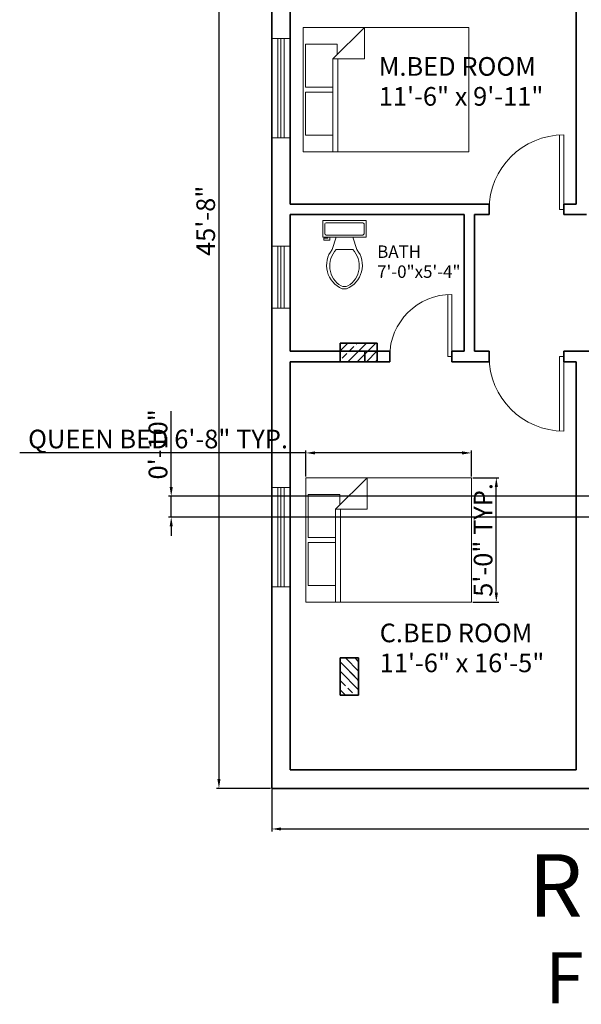
# Model space of a CAD drawing. Units: inches. Extents: x 2081 to 4786, y 1256 to 3802.
# Tile 1 of 7: x 2081 to 2352, y 1329 to 1804. Entities that reach past the tile are written whole.
import ezdxf

# ---------------------------------------------------------------- set-up
doc = ezdxf.new("R2010")
doc.units = ezdxf.units.IN
for name, color, linetype, lineweight in [('A-ANNO-DIMS', 18, 'Continuous', 18), ('A-ANNO-TITL', 18, 'Continuous', 35), ('A-AREA-IDEN', 18, 'Continuous', 18), ('A-COLS', 1, 'Continuous', 35), ('A-DOOR', 5, 'Continuous', 18), ('A-FLOR-FIXT', 18, 'Continuous', 18), ('A-FURN', 5, 'Continuous', 18), ('A-GLAZ', 11, 'Continuous', 18), ('A-WALL', 7, 'Continuous', 35)]:
    doc.layers.add(name, color=color, linetype=linetype, lineweight=lineweight)
doc.styles.get("Standard").update_dxf_attribs({"font": 'arial.ttf'})
doc.dimstyles.new('ISO-25', dxfattribs={"dimtxt": 9, "dimasz": 4.5, "dimexe": 1.25, "dimexo": 0.625, "dimtad": 1, "dimdec": 0, "dimlunit": 3, "dimtxsty": 'Standard', "dimcen": 2.5, "dimadec": 0, "dimazin": 0, "dimtfac": 1, "dimtdec": 0, "dimtmove": 0, "dimatfit": 3, "dimfxl": 1, "dimarcsym": 0})
pattern_1 = [(135, (1916.44, -3174.735), (-13.47038, -13.47038), []), (135, (1916.44, -3170.245), (-13.47038, -13.47038), []), (135, (1916.44, -3165.755), (-13.47038, -13.47038), []), (135, (1916.44, -3161.265), (-13.47038, -13.47038), [])]

# ---------------------------------------------------------------- blocks, each defined once
blk = doc.blocks.new('Bed - Queen')
for p, q in [((0, -80.00003), (0, 0)), ((0, 0), (59.99999, 0)), ((59.99999, 0), (59.99999, -80.00003)), ((7.99999, -1.2), (28.79998, -1.2)), ((7.99999, -14.4), (7.99999, -1.2)), ((28.79998, -1.2), (28.79998, -14.4)), ((31.19999, -1.2), (51.99999, -1.2)), ((31.19999, -14.4), (31.19999, -1.2)), ((51.99999, -1.2), (51.99999, -16.4)), ((0, -14.4), (44.8, -14.4)), ((44.8, -16.8), (0, -16.8)), ((59.99999, -29.6), (44.8, -14.4)), ((44.8, -14.4), (44.8, -29.6)), ((51.99999, -16.4), (46.79936, -16.4)), ((44.8, -29.6), (59.99999, -29.6)), ((59.99999, -80.00003), (0, -80.00003))]:
    blk.add_line(p, q)
blk = doc.blocks.new('Toilet - top')
for p, q in [((9.5, -6), (9.5, -2)), ((-10, -8.5), (-8, -8.5)), ((-10, -9.5), (-10, -8.5)), ((-7, -9.5), (-10, -9.5)), ((-8, -8.5), (-8, -8)), ((-7, -8), (-7, -9.5)), ((-4, -8), (-6, -14)), ((4, -8), (6, -14)), ((4, -14), (-4, -14))]:
    blk.add_line(p, q)
blk.add_lwpolyline([(10.5, -8), (10.5, 0), (-10.5, 0), (-10.5, -8)], close=True)
for points in [[(-9.5, -2), (-9.5, -6)], [(8.5, -1), (-8.5, -1)], [(-8.5, -7), (8.5, -7)]]:
    blk.add_lwpolyline(points)
for centre, radius, start, end in [((-8.62, -1.88), 0.884, 81.8699, 188.1301), ((8.62, -1.88), 0.884, 351.8699, 98.1301), ((-8.62, -6.12), 0.884, 171.8699, 278.1301), ((8.62, -6.12), 0.884, 261.8699, 8.1301), ((3.52, -21.58), 12.17, 141.4691, 247.9714), ((4.2, -21.82), 11.33, 136.3677, 238.9468), ((-3.52, -21.58), 12.17, 292.0284, 38.5307), ((-4.2, -21.82), 11.33, 301.053, 43.6321), ((0, -27.88), 4, 245.7318, 294.2682), ((0, -29), 4, 254.8605, 285.1395)]:
    blk.add_arc(centre, radius, start, end)
blk = doc.blocks.new('*D25')
at = {"layer": 'A-ANNO-DIMS', "color": 0, "lineweight": -2, "transparency": 16777216}
for p, q in [((2202.36, 1981.17), (2176.26, 1981.17)), ((2177.51, 1976.67), (2177.51, 1437.67)), ((2202.36, 1433.17), (2176.26, 1433.17))]:
    blk.add_line(p, q, dxfattribs=at)
at = {"layer": 'A-ANNO-DIMS', "color": 0, "transparency": 16777216}
for points in [[(2176.76, 1976.67), (2178.26, 1976.67), (2177.51, 1981.17)], [(2176.76, 1437.67), (2178.26, 1437.67), (2177.51, 1433.17)]]:
    blk.add_solid(points, dxfattribs=at)
at = {"layer": 'Defpoints', "color": 0, "transparency": 16777216}
for p in [(2202.98, 1981.17), (2177.51, 1433.17), (2202.98, 1433.17)]:
    blk.add_point(p, dxfattribs=at)
at = {"layer": 'A-ANNO-DIMS', "color": 0, "transparency": 16777216, "insert": (2172.29, 1707.17), "char_height": 9, "attachment_point": 5, "rotation": 90}
blk.add_mtext('45\'-8"', dxfattribs=at)
blk = doc.blocks.new('*D26')
at = {"layer": 'A-ANNO-DIMS', "color": 0, "lineweight": -2, "transparency": 16777216}
for p, q in [((2202.98, 1432.55), (2202.98, 1412.32)), ((3062.98, 1432.55), (3062.98, 1412.32)), ((2207.48, 1413.57), (3058.48, 1413.57))]:
    blk.add_line(p, q, dxfattribs=at)
at = {"layer": 'A-ANNO-DIMS', "color": 0, "transparency": 16777216}
for points in [[(2207.48, 1414.32), (2207.48, 1412.82), (2202.98, 1413.57)], [(3058.48, 1414.32), (3058.48, 1412.82), (3062.98, 1413.57)]]:
    blk.add_solid(points, dxfattribs=at)
at = {"layer": 'Defpoints', "color": 0, "transparency": 16777216}
for p in [(2202.98, 1433.17), (3062.98, 1433.17), (3062.98, 1413.57)]:
    blk.add_point(p, dxfattribs=at)
at = {"layer": 'A-ANNO-DIMS', "color": 0, "transparency": 16777216, "insert": (2632.98, 1418.79), "char_height": 9, "attachment_point": 5}
blk.add_mtext('71\'-8"', dxfattribs=at)
blk = doc.blocks.new('DOOR-SINGLE-36IN')
for p, q in [((34, 36), (34, 0)), ((36, 36), (36, 0)), ((36, 0), (34, 0))]:
    blk.add_line(p, q)
blk.add_arc((36, 0), 36, 90, 180)
blk = doc.blocks.new('DOOR-SINGLE-30IN')
for p, q in [((0, 30), (30, 30)), ((30, 30), (30, 28)), ((0, 28), (30, 28))]:
    blk.add_line(p, q)
blk.add_arc((30, 30), 30, 180, 270)
blk = doc.blocks.new('WINDOW-48IN')
for p, q in [((0, 0), (0, 9)), ((0, 9), (4, 9)), ((48, 6), (0, 6)), ((4, 9), (48, 9)), ((48, 0), (48, 9)), ((48, 4.5), (0, 4.5)), ((48, 3), (0, 3)), ((48, 0), (0, 0))]:
    blk.add_line(p, q)
blk = doc.blocks.new('WINDOW-30IN')
for p, q in [((0, 0), (0, 30)), ((0, 30), (9, 30)), ((3, 0), (3, 30)), ((4.5, 0), (4.5, 30)), ((6, 0), (6, 30)), ((9, 30), (9, 0)), ((9, 0), (0, 0))]:
    blk.add_line(p, q)
blk = doc.blocks.new('COLUMN-9X18IN')
h = blk.add_hatch()
h.set_pattern_fill('ANSI34', color=256, angle=90)
h.set_pattern_definition(pattern_1)
h.paths.add_polyline_path([(9, 18), (0, 18), (0, 0), (9, 0)])
h = blk.add_hatch()
h.set_pattern_fill('ANSI34', color=256, angle=90)
h.set_pattern_definition(pattern_1)
h.paths.add_polyline_path([(9, 18), (0, 18), (0, 0), (9, 0)])
h = blk.add_hatch()
h.set_pattern_fill('ANSI34', color=256, angle=90)
h.set_pattern_definition(pattern_1)
h.paths.add_polyline_path([(9, 18), (0, 18), (0, 0), (9, 0)])
h = blk.add_hatch()
h.set_pattern_fill('ANSI33', color=256, angle=90)
h.set_pattern_definition([(135, (1916.44, -3174.7355), (-4.490128, -4.490128), []), (135, (1916.44, -3170.2454), (-4.490128, -4.490128), [3.175, -1.5875])])
h.paths.add_polyline_path([(0, 0), (9, 0), (9, 18), (0, 18)])
for p, q in [((0, 0), (0, 18)), ((0, 18), (9, 18)), ((9, 18), (9, 0)), ((9, 0), (0, 0))]:
    blk.add_line(p, q)
blk = doc.blocks.new('*D37')
at = {"layer": 'A-ANNO-DIMS', "color": 0, "lineweight": -2, "transparency": 16777216}
for p, q in [((2219.45, 1595.12), (2081.31, 1595.12)), ((2219.45, 1583.74), (2219.45, 1596.37)), ((2294.95, 1595.12), (2223.95, 1595.12)), ((2299.45, 1583.74), (2299.45, 1596.37))]:
    blk.add_line(p, q, dxfattribs=at)
at = {"layer": 'A-ANNO-DIMS', "color": 0, "transparency": 16777216}
for points in [[(2223.95, 1595.87), (2223.95, 1594.37), (2219.45, 1595.12)], [(2294.95, 1595.87), (2294.95, 1594.37), (2299.45, 1595.12)]]:
    blk.add_solid(points, dxfattribs=at)
at = {"layer": 'Defpoints', "color": 0, "transparency": 16777216}
for p in [(2219.45, 1595.12), (2219.45, 1583.12), (2299.45, 1583.12)]:
    blk.add_point(p, dxfattribs=at)
at = {"layer": 'A-ANNO-DIMS', "color": 0, "transparency": 16777216, "insert": (2148.13, 1600.67), "char_height": 9, "attachment_point": 5}
blk.add_mtext('QUEEN BED 6\'-8" TYP.', dxfattribs=at)
blk = doc.blocks.new('*D38')
at = {"layer": 'A-ANNO-DIMS', "color": 0, "lineweight": -2, "transparency": 16777216}
for p, q in [((2300.08, 1583.12), (2312.7, 1583.12)), ((2311.45, 1527.62), (2311.45, 1578.62)), ((2300.08, 1523.12), (2312.7, 1523.12))]:
    blk.add_line(p, q, dxfattribs=at)
at = {"layer": 'A-ANNO-DIMS', "color": 0, "transparency": 16777216}
for points in [[(2310.7, 1578.62), (2312.2, 1578.62), (2311.45, 1583.12)], [(2310.7, 1527.62), (2312.2, 1527.62), (2311.45, 1523.12)]]:
    blk.add_solid(points, dxfattribs=at)
at = {"layer": 'Defpoints', "color": 0, "transparency": 16777216}
for p in [(2299.45, 1583.12), (2311.45, 1583.12), (2299.45, 1523.12)]:
    blk.add_point(p, dxfattribs=at)
at = {"layer": 'A-ANNO-DIMS', "color": 0, "transparency": 16777216, "insert": (2306.23, 1553.12), "char_height": 9, "attachment_point": 5, "rotation": 90}
blk.add_mtext('5\'-0" TYP.', dxfattribs=at)
blk = doc.blocks.new('*D60')
at = {"layer": 'A-ANNO-DIMS', "color": 0, "lineweight": -2, "transparency": 16777216}
for p, q in [((2358.89, 1801.88), (2358.89, 1811.5)), ((2380.23, 1801.88), (2380.23, 1811.5)), ((2358.89, 1810.25), (2278.16, 1810.25)), ((2375.73, 1810.25), (2363.39, 1810.25))]:
    blk.add_line(p, q, dxfattribs=at)
at = {"layer": 'A-ANNO-DIMS', "color": 0, "transparency": 16777216}
for points in [[(2363.39, 1811), (2363.39, 1809.5), (2358.89, 1810.25)], [(2375.73, 1811), (2375.73, 1809.5), (2380.23, 1810.25)]]:
    blk.add_solid(points, dxfattribs=at)
at = {"layer": 'Defpoints', "color": 0, "transparency": 16777216}
for p in [(2358.89, 1810.25), (2358.89, 1801.25), (2380.23, 1801.25)]:
    blk.add_point(p, dxfattribs=at)
at = {"layer": 'A-ANNO-DIMS', "color": 0, "transparency": 16777216, "insert": (2316.28, 1815.53), "char_height": 9, "attachment_point": 5}
blk.add_mtext('1\'-9 1/2" TYP.', dxfattribs=at)
blk = doc.blocks.new('*D81')
at = {"layer": 'A-ANNO-DIMS', "color": 0, "lineweight": -2, "transparency": 16777216}
for p, q in [((2154.48, 1578.67), (2154.48, 1615.34)), ((2684.36, 1574.17), (2153.23, 1574.17)), ((2154.48, 1564.17), (2154.48, 1574.17)), ((2684.36, 1564.17), (2153.23, 1564.17)), ((2154.48, 1559.67), (2154.48, 1555.17))]:
    blk.add_line(p, q, dxfattribs=at)
at = {"layer": 'A-ANNO-DIMS', "color": 0, "transparency": 16777216}
for points in [[(2153.73, 1578.67), (2155.23, 1578.67), (2154.48, 1574.17)], [(2153.73, 1559.67), (2155.23, 1559.67), (2154.48, 1564.17)]]:
    blk.add_solid(points, dxfattribs=at)
at = {"layer": 'Defpoints', "color": 0, "transparency": 16777216}
for p in [(2154.48, 1574.17), (2684.98, 1574.17), (2684.98, 1564.17)]:
    blk.add_point(p, dxfattribs=at)
at = {"layer": 'A-ANNO-DIMS', "color": 0, "transparency": 16777216, "insert": (2149.26, 1599.26), "char_height": 9, "attachment_point": 5, "rotation": 90}
blk.add_mtext('0\'-10"', dxfattribs=at)

msp = doc.modelspace()

# ---------------------------------------------------------------- linework, layer by layer
at = {"layer": 'A-WALL'}
for p, q in [((2202.98, 1981.17), (2202.98, 1433.17)), ((2211.98, 1715.17), (2211.98, 1834.17)), ((2349.98, 1715.17), (2349.98, 1834.17)), ((2211.98, 1715.17), (2307.98, 1715.17)), ((2307.98, 1710.17), (2307.98, 1715.17)), ((2343.98, 1710.17), (2343.98, 1715.17)), ((2343.98, 1715.17), (2349.98, 1715.17)), ((2211.98, 1710.17), (2295.98, 1710.17)), ((2211.98, 1644.17), (2211.98, 1710.17)), ((2295.98, 1644.17), (2295.98, 1710.17)), ((2300.98, 1644.17), (2300.98, 1710.17)), ((2300.98, 1710.17), (2307.98, 1710.17)), ((2343.98, 1710.17), (2354.98, 1710.17)), ((2211.98, 1644.17), (2259.98, 1644.17)), ((2247.98, 1639.17), (2247.98, 1644.17)), ((2259.98, 1644.17), (2259.98, 1639.17)), ((2289.98, 1639.17), (2289.98, 1644.17)), ((2289.98, 1644.17), (2295.98, 1644.17)), ((2300.98, 1644.17), (2307.98, 1644.17)), ((2307.98, 1639.17), (2307.98, 1644.17)), ((2343.98, 1639.17), (2343.98, 1644.17)), ((2343.98, 1644.17), (2429.98, 1644.17)), ((2211.98, 1442.17), (2211.98, 1639.17)), ((2211.98, 1639.17), (2259.98, 1639.17)), ((2289.98, 1639.17), (2307.98, 1639.17)), ((2343.98, 1639.17), (2349.98, 1639.17)), ((2349.98, 1442.17), (2349.98, 1639.17)), ((2349.98, 1442.17), (2211.98, 1442.17)), ((3062.98, 1433.17), (2202.98, 1433.17))]:
    msp.add_line(p, q, dxfattribs=at)

# ---------------------------------------------------------------- block references
at = {"layer": 'A-COLS', "rotation": 269.9999999999957}
msp.add_blockref('COLUMN-9X18IN', (2235.98, 1648.17), dxfattribs=at)
at = {"layer": 'A-COLS'}
msp.add_blockref('COLUMN-9X18IN', (2235.98, 1478.17), dxfattribs=at)
at = {"layer": 'A-DOOR'}
msp.add_blockref('DOOR-SINGLE-36IN', (2307.98, 1712.67), dxfattribs=at)
at = {"layer": 'A-DOOR', "rotation": 270}
msp.add_blockref('DOOR-SINGLE-30IN', (2259.98, 1671.67), dxfattribs=at)
at = {"layer": 'A-DOOR', "extrusion": (0, 0, -1), "zscale": -1, "rotation": 180}
msp.add_blockref('DOOR-SINGLE-36IN', (-2307.98, 1641.67), dxfattribs=at)
at = {"layer": 'A-FLOR-FIXT'}
msp.add_blockref('Toilet - top', (2238.13, 1707.27), dxfattribs=at)
at = {"layer": 'A-FURN', "rotation": 90}
for p in [(2218.18, 1740.5), (2219.45, 1523.12)]:
    msp.add_blockref('Bed - Queen', p, dxfattribs=at)
at = {"layer": 'A-GLAZ'}
for p, rotation in [((2202.98, 1795.16), 269.9999999999992), ((2202.98, 1578.42), 269.9999999999987)]:
    msp.add_blockref('WINDOW-48IN', p, dxfattribs=dict(at, rotation=rotation))
msp.add_blockref('WINDOW-30IN', (2202.98, 1665.01), dxfattribs=at)

# ---------------------------------------------------------------- texts
at = {"layer": 'A-ANNO-TITL'}
for s, height, p in [('RESIDENTIAL APARTMENT', 30.1152, (2327.01, 1371.26)), ('FIRST FLOOR ', 24.6271, (2335.08, 1329.36))]:
    msp.add_text(s, height=height, dxfattribs=at).set_placement(p)
at = {"layer": 'A-AREA-IDEN'}
for s, height, p in [('M.BED ROOM', 9, (2254.69, 1777.22)), ('11\'-6" x 9\'-11"', 9, (2254.69, 1762.76)), ('BATH', 6, (2253.91, 1689.28)), ('7\'-0"x5\'-4"', 6, (2253.91, 1679.64)), ('C.BED ROOM', 9, (2255.13, 1503.72)), ('11\'-6" x 16\'-5"', 9, (2255.13, 1489.26))]:
    msp.add_text(s, height=height, dxfattribs=at).set_placement(p)

# ---------------------------------------------------------------- dimensions: what is measured, and where the dimension line sits
at = {"layer": 'A-ANNO-DIMS'}
for base, p1, p2, override, picture, middle in [((2177.51, 1433.17), (2202.98, 1981.17), (2202.98, 1433.17), {"dimclrd": 0, "dimclre": 0, "dimclrt": 0}, '*D25', (2172.29, 1707.17)), ((2154.48, 1574.17), (2684.98, 1564.17), (2684.98, 1574.17), {"dimdec": 1, "dimlfac": 1, "dimrnd": 0, "dimzin": 1, "dimdsep": 46, "dimlunit": 4, "dimfrac": 2}, '*D81', (2149.26, 1599.26))]:
    dim = msp.add_linear_dim(base=base, p1=p1, p2=p2, angle=90, dimstyle='ISO-25', override=override, dxfattribs=at)
    dim.commit()
    dim.dimension.update_dxf_attribs({"geometry": picture, "text_midpoint": middle})
for base, p1, p2, angle, text, picture, middle in [((2358.89, 1810.25), (2380.23, 1801.25), (2358.89, 1801.25), 180, '<> TYP.', '*D60', (2316.28, 1815.53)), ((2219.45, 1595.12), (2299.45, 1583.12), (2219.45, 1583.12), 180, 'QUEEN BED <> TYP.', '*D37', (2148.13, 1600.67)), ((2311.45, 1583.12), (2299.45, 1523.12), (2299.45, 1583.12), 90, '<> TYP.', '*D38', (2306.23, 1553.12))]:
    dim = msp.add_linear_dim(base=base, p1=p1, p2=p2, angle=angle, text=text, dimstyle='ISO-25', override={"dimdec": 1, "dimlfac": 1, "dimrnd": 0, "dimzin": 1, "dimdsep": 46, "dimlunit": 4, "dimfrac": 2}, dxfattribs=at)
    dim.commit()
    dim.dimension.update_dxf_attribs({"geometry": picture, "text_midpoint": middle})
dim = msp.add_linear_dim(base=(3062.98, 1413.57), p1=(2202.98, 1433.17), p2=(3062.98, 1433.17), dimstyle='ISO-25', override={"dimclrd": 0, "dimclre": 0, "dimclrt": 0}, dxfattribs=at)
dim.commit()
dim.dimension.update_dxf_attribs({"geometry": '*D26', "text_midpoint": (2632.98, 1418.79)})

doc.saveas('drawing.dxf')
